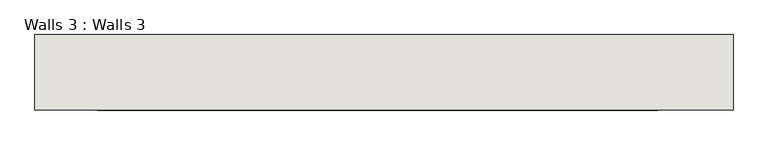
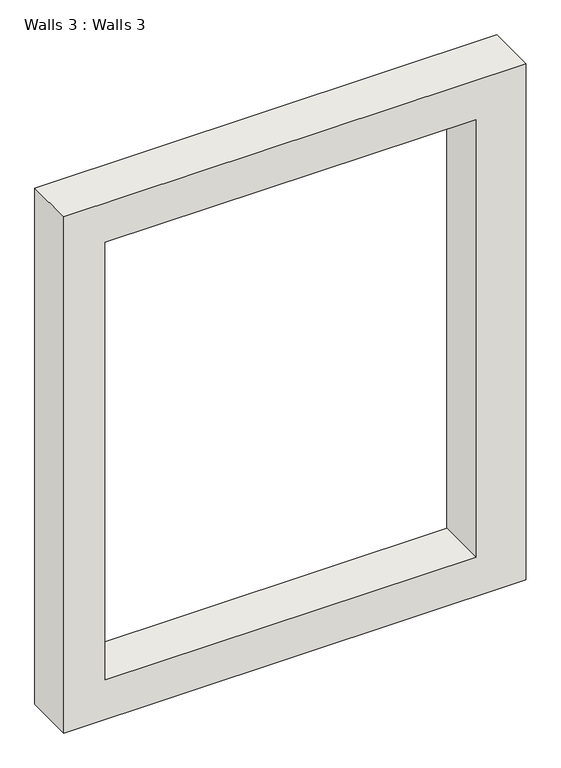
"""IFC4 building model written with IfcOpenShell, lengths in millimetres: wall geometry, Walls 3 : Walls 3."""

from ifc_helpers import new_model, si_unit, frame, origin, place, context, project, spatial, polyline, outline, extrude, source, transform, mapped, element, save


def walls_3_walls_3_01008c03(model_context):
    return source(origin(), model_context, "Body", "SweptSolid", [
        extrude(outline(polyline([(2768.6, -6524.8569651), (2768.6, -3705.4569651), (6096.0, -3705.4569651), (6096.0, -6524.8569651), (2768.6, -6524.8569651)]), holes=[polyline([(3022.6, -6270.8569651), (5842.0, -6270.8569651), (5842.0, -4010.2569651), (3022.6, -4010.2569651), (3022.6, -6270.8569651)])]), frame((0.0, 146.7055142, 0.0), z_axis=(0.0, 1.0, 0.0), x_axis=(0.0, 0.0, 1.0)), (0.0, 0.0, 1.0), 304.8),
    ])


if __name__ == "__main__":
    model = new_model("IFC4")
    model_context = context("Model", 3, world=origin())
    ifc_project = project(units=[si_unit("LENGTHUNIT", "METRE", prefix="MILLI")], contexts=[model_context])
    site = spatial("IfcSite", under=ifc_project)
    building = spatial("IfcBuilding", under=site)
    placement = place(None, origin())
    walls_3_walls_3_shape = walls_3_walls_3_01008c03(model_context)
    element("IfcWall", 1, ObjectType="Walls 3 : Walls 3", at=placement, inside=building, context=model_context, shape_type="MappedRepresentation", body=[
        mapped(walls_3_walls_3_shape, transform((0.0, 0.0, 0.0), x_axis=(1.0, 0.0, 0.0), y_axis=(0.0, 1.0, 0.0), z_axis=(0.0, 0.0, 1.0))),
    ])
    save(model, "model.ifc")

# Revit data of these elements
# Element 1 (IfcWall, "Walls 3 : Walls 3")
#   Materials on its faces: "1 wall white", "Default Wall"
# Materials
#   "1 wall white": class "Generic", colour RGB 244 245 241, transparency 0, Cost = 0
#   "Default Wall": colour RGB 128 128 128, transparency 0, Cost = 0
